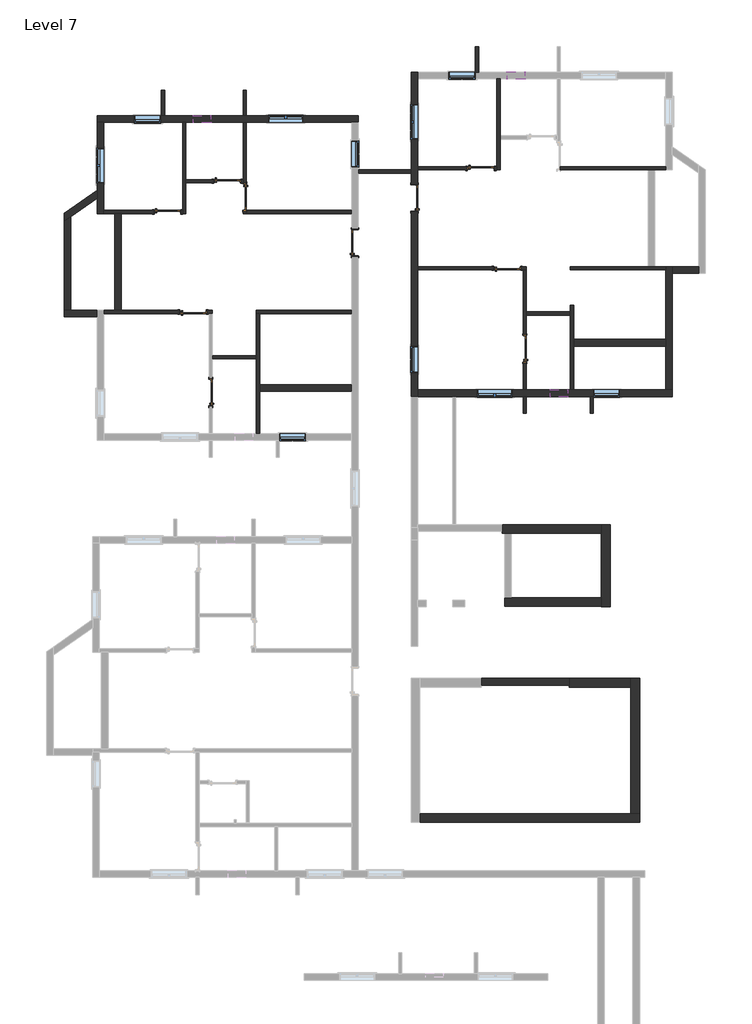
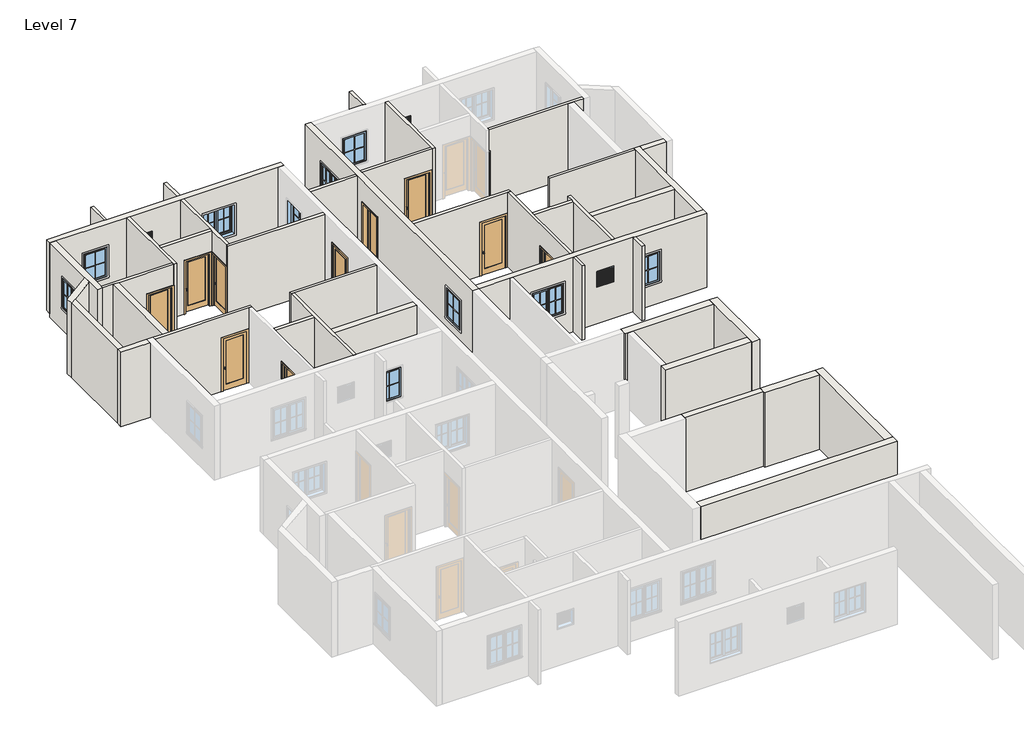
# One storey, part 5 of 7: 42 walls, 13 windows, 10 doors.
# Revit data of these elements (continued)
# Element 54 (IfcWindow, "Window-Awning-Single : 36\" x 48\"") (continued)
#   Interior Wall Closure = 0' - 2 1/4"
#   Frame Extension = 0' - 0 1/4"
#   Exterior Wall Closure = 0' - 1 1/4"
#   Interior Trim Visibility = yes
#   Exterior Trim Visibility = yes
#   Phase Created = New Construction
#   Materials on its faces: "Wood - Stained", "Glass", "Clad - White"
# Element 55 (IfcWindow, "Window-Awning-Single : 36\" x 48\"")
#   Mark = "152"
#   Window Inset = 0' - 0"
#   Interior Wall Closure = 0' - 2 1/4"
#   Frame Extension = 0' - 0 1/4"
#   Exterior Wall Closure = 0' - 1 1/4"
#   Interior Trim Visibility = yes
#   Exterior Trim Visibility = yes
#   Phase Created = New Construction
#   Materials on its faces: "Wood - Stained", "Glass", "Clad - White"
# Element 56 (IfcWindow, "Window-Awning-Single : 36\" x 48\"")
#   Mark = "154"
#   Window Inset = 0' - 0"
#   Interior Wall Closure = 0' - 2 1/4"
#   Frame Extension = 0' - 0 1/4"
#   Exterior Wall Closure = 0' - 1 1/4"
#   Interior Trim Visibility = yes
#   Exterior Trim Visibility = yes
#   Phase Created = New Construction
#   Materials on its faces: "Wood - Stained", "Glass", "Clad - White"
# Element 57 (IfcWindow, "Window-Awning-Single : 36\" x 48\"")
#   Mark = "156"
#   Window Inset = 0' - 0"
#   Interior Wall Closure = 0' - 2 1/4"
#   Frame Extension = 0' - 0 1/4"
#   Exterior Wall Closure = 0' - 1 1/4"
#   Interior Trim Visibility = yes
#   Exterior Trim Visibility = yes
#   Phase Created = New Construction
#   Materials on its faces: "Wood - Stained", "Glass", "Clad - White"
# Element 58 (IfcWindow, "Window-Awning-Single : 36\" x 48\"")
#   Mark = "157"
#   Window Inset = 0' - 0"
#   Interior Wall Closure = 0' - 2 1/4"
#   Frame Extension = 0' - 0 1/4"
#   Exterior Wall Closure = 0' - 1 1/4"
#   Interior Trim Visibility = yes
#   Exterior Trim Visibility = yes
#   Phase Created = New Construction
#   Materials on its faces: "Wood - Stained", "Glass", "Clad - White"
# Element 59 (IfcWindow, "Window-Casement-Double : 4' x 4'")
#   Mark = "166"
#   Window Inset = 0' - 0"
#   Interior Wall Closure = 0' - 2 1/4"
#   Frame Extension = 0' - 0 1/4"
#   Exterior Wall Closure = 0' - 1 1/4"
#   Interior Trim Visibility = yes
#   Exterior Trim Visibility = yes
#   Phase Created = New Construction
#   Materials on its faces: "Wood - Stained", "Glass", "Clad - White"
# Element 60 (IfcWindow, "Window-Casement-Double : 4' x 4'")
#   Mark = "167"
#   Window Inset = 0' - 0"
#   Interior Wall Closure = 0' - 2 1/4"
#   Frame Extension = 0' - 0 1/4"
#   Exterior Wall Closure = 0' - 1 1/4"
#   Interior Trim Visibility = yes
#   Exterior Trim Visibility = yes
#   Phase Created = New Construction
#   Materials on its faces: "Wood - Stained", "Glass", "Clad - White"
# Element 61 (IfcWindow, "Window-Casement-Double : 4' x 4'")
#   Mark = "169"
#   Window Inset = 0' - 0"
#   Interior Wall Closure = 0' - 2 1/4"
#   Frame Extension = 0' - 0 1/4"
#   Exterior Wall Closure = 0' - 1 1/4"
#   Interior Trim Visibility = yes
#   Exterior Trim Visibility = yes
#   Phase Created = New Construction
#   Materials on its faces: "Wood - Stained", "Glass", "Clad - White"
# Element 62 (IfcWindow, "Window-Casement-Double : 4' x 4'")
#   Mark = "171"
#   Window Inset = 0' - 0"
#   Interior Wall Closure = 0' - 2 1/4"
#   Frame Extension = 0' - 0 1/4"
#   Exterior Wall Closure = 0' - 1 1/4"
#   Interior Trim Visibility = yes
#   Exterior Trim Visibility = yes
#   Phase Created = New Construction
#   Materials on its faces: "Wood - Stained", "Glass", "Clad - White"
# Element 63 (IfcWindow, "Window-Louvers : 24\" x 24\"")
#   Mark = "133"
#   Blade Width = 1' - 10 1/2"
#   Phase Created = New Construction
#   Materials on its faces: "Birch"
# Element 64 (IfcWindow, "Window-Louvers : 24\" x 24\"")
#   Mark = "135"
#   Blade Width = 1' - 10 1/2"
#   Phase Created = New Construction
#   Materials on its faces: "Birch"
# Element 65 (IfcWindow, "Window-Louvers : 24\" x 24\"")
#   Mark = "136"
#   Blade Width = 1' - 10 1/2"
#   Phase Created = New Construction
#   Materials on its faces: "Birch"
# Materials
#   "Cherry": class "Wood", colour RGB 226 177 128, transparency 0, Description = "Prunus Serotina", Cost = 0
#   "Aluminum": class "Metal", colour RGB 247 247 247, transparency 0, Description = "Aluminum 6061", Cost = 0
#   "Wood - Stained": class "Wood", colour RGB 224 178 126, transparency 0, Cost = 0
#   "Glass": class "Glass", colour RGB 0 128 192, transparency 0.75, Description = "Soda Lime Glass", Cost = 0
#   "Clad - White": class "Wood", colour RGB 242 242 238, transparency 0, Cost = 0
#   "Birch": class "Wood", colour RGB 224 178 126, transparency 0, Description = "Betula Alleghaniensis", Cost = 0
#   "Default Wall": colour RGB 128 128 128, transparency 0, Cost = 0
